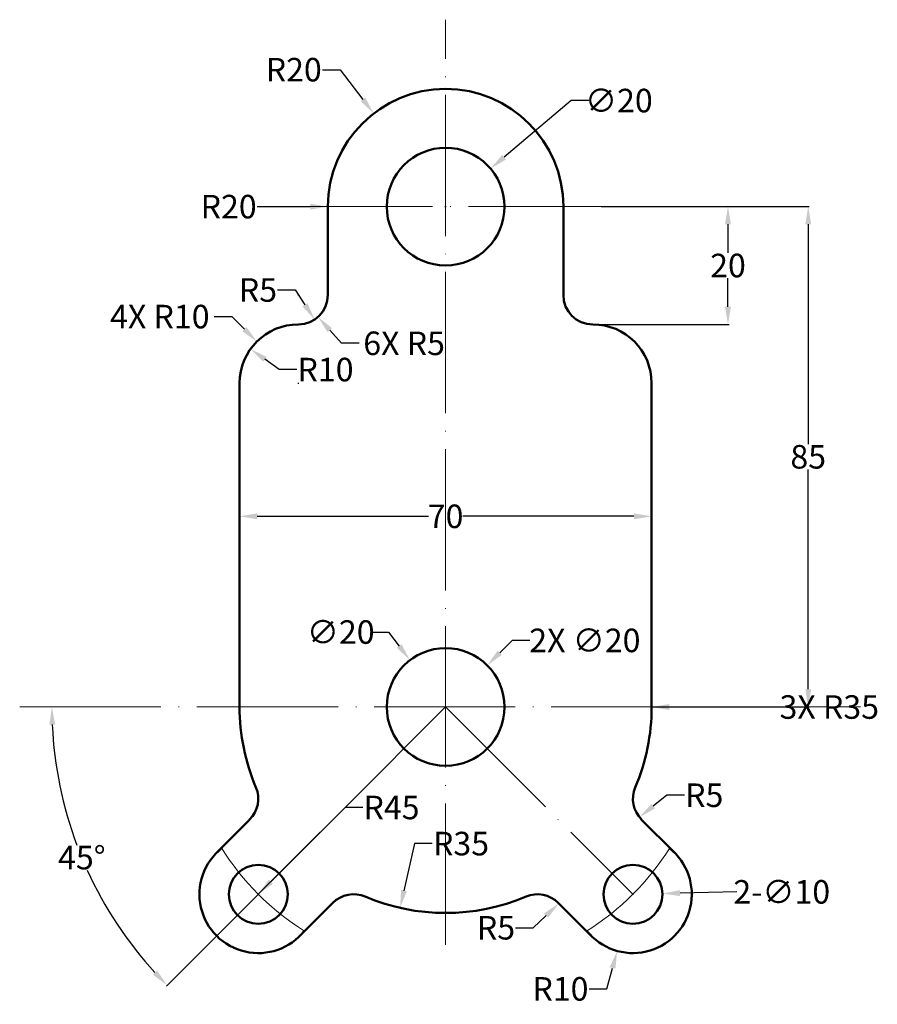
# Model space of a CAD drawing. Units: inches. Extents: x 93 to 239, y 45 to 212.
import ezdxf

# ---------------------------------------------------------------- set-up
doc = ezdxf.new("R2010")
doc.units = ezdxf.units.IN
doc.header["$MEASUREMENT"] = 0
doc.linetypes.add('ACAD_ISO04W100', pattern=[30, 24, -3, 0, -3])
for name, color, linetype, lineweight in [('M-CNTR', 4, 'ACAD_ISO04W100', 18), ('M-DIMS', 2, 'Continuous', 25), ('M-OUTL', 7, 'Continuous', 50)]:
    doc.layers.add(name, color=color, linetype=linetype, lineweight=lineweight)
doc.styles.get("Standard").update_dxf_attribs({"font": 'arial.ttf'})
doc.dimstyles.get("Standard").update_dxf_attribs({"dimtxt": 4, "dimasz": 3, "dimexe": 0.18, "dimexo": 0.0625, "dimgap": 0.09, "dimtad": 0, "dimtih": 1, "dimtoh": 1, "dimdec": 0, "dimzin": 0, "dimdsep": 46, "dimtxsty": 'Standard', "dimcen": 0.09, "dimadec": 0, "dimazin": 0, "dimtfac": 1, "dimtdec": 0, "dimtofl": 0, "dimtmove": 0, "dimatfit": 3, "dimfxl": 1, "dimtolj": 1, "dimtzin": 0, "dimarcsym": 0})

# ---------------------------------------------------------------- blocks, each defined once
blk = doc.blocks.new('*D1')
at = {"layer": 'Defpoints', "color": 0, "transparency": 16777216}
for p in [(192.05, 180.39), (190.67, 160.39), (213.64, 160.39)]:
    blk.add_point(p, dxfattribs=at)
at = {"layer": 'M-DIMS', "color": 0, "lineweight": -2, "transparency": 16777216}
for p, q in [((192.11, 180.39), (213.82, 180.39)), ((213.64, 177.39), (213.64, 172.53)), ((213.64, 163.39), (213.64, 168.26)), ((190.73, 160.39), (213.82, 160.39))]:
    blk.add_line(p, q, dxfattribs=at)
at = {"layer": 'M-DIMS', "color": 0, "transparency": 16777216}
for points in [[(213.14, 177.39), (214.14, 177.39), (213.64, 180.39)], [(213.14, 163.39), (214.14, 163.39), (213.64, 160.39)]]:
    blk.add_solid(points, dxfattribs=at)
at = {"layer": 'M-DIMS', "color": 0, "transparency": 16777216, "insert": (213.64, 170.39), "char_height": 4, "attachment_point": 5}
blk.add_mtext('\\A1;20', dxfattribs=at)
blk = doc.blocks.new('*D2')
at = {"layer": 'Defpoints', "color": 0, "transparency": 16777216}
for p in [(192.05, 180.39), (200.67, 95.39), (227.27, 95.39)]:
    blk.add_point(p, dxfattribs=at)
at = {"layer": 'M-DIMS', "color": 0, "lineweight": -2, "transparency": 16777216}
for p, q in [((192.11, 180.39), (227.45, 180.39)), ((227.27, 177.39), (227.27, 140.03)), ((227.27, 98.39), (227.27, 135.76)), ((200.73, 95.39), (227.45, 95.39))]:
    blk.add_line(p, q, dxfattribs=at)
at = {"layer": 'M-DIMS', "color": 0, "transparency": 16777216}
for points in [[(226.77, 177.39), (227.77, 177.39), (227.27, 180.39)], [(226.77, 98.39), (227.77, 98.39), (227.27, 95.39)]]:
    blk.add_solid(points, dxfattribs=at)
at = {"layer": 'M-DIMS', "color": 0, "transparency": 16777216, "insert": (227.27, 137.89), "char_height": 4, "attachment_point": 5}
blk.add_mtext('\\A1;85', dxfattribs=at)
blk = doc.blocks.new('*D3')
at = {"layer": 'Defpoints', "color": 0, "transparency": 16777216}
for p in [(197.49, 63.57), (194.82, 53.93)]:
    blk.add_point(p, dxfattribs=at)
at = {"layer": 'M-DIMS', "color": 0, "lineweight": -2, "transparency": 16777216}
for p, q in [((197.4, 63.57), (197.58, 63.57)), ((197.49, 63.48), (197.49, 63.66)), ((193.05, 47.5), (194.02, 51.04)), ((190.05, 47.5), (193.05, 47.5))]:
    blk.add_line(p, q, dxfattribs=at)
at = {"layer": 'M-DIMS', "color": 0, "transparency": 16777216}
blk.add_solid([(193.54, 51.18), (194.51, 50.91), (194.82, 53.93)], dxfattribs=at)
at = {"layer": 'M-DIMS', "color": 0, "transparency": 16777216, "insert": (185.18, 47.5), "char_height": 4, "attachment_point": 5}
blk.add_mtext('\\A1;R10', dxfattribs=at)
blk = doc.blocks.new('*D4')
at = {"layer": 'Defpoints', "color": 0, "transparency": 16777216}
for p in [(184.9, 62.02), (181.28, 58.57)]:
    blk.add_point(p, dxfattribs=at)
at = {"layer": 'M-DIMS', "color": 0, "lineweight": -2, "transparency": 16777216}
for p, q in [((180.56, 57.88), (182.73, 59.95)), ((177.56, 57.88), (180.56, 57.88))]:
    blk.add_line(p, q, dxfattribs=at)
blk.add_arc((181.28, 58.57), 5, 41.564, 44.2838, dxfattribs=at)
at = {"layer": 'M-DIMS', "color": 0, "transparency": 16777216}
blk.add_solid([(182.39, 60.31), (183.08, 59.58), (184.9, 62.02)], dxfattribs=at)
at = {"layer": 'M-DIMS', "color": 0, "transparency": 16777216, "insert": (174.23, 57.88), "char_height": 4, "attachment_point": 5}
blk.add_mtext('\\A1;R5', dxfattribs=at)
blk = doc.blocks.new('*D5')
at = {"layer": 'Defpoints', "color": 0, "transparency": 16777216}
for p in [(165.67, 95.39), (157.93, 61.26)]:
    blk.add_point(p, dxfattribs=at)
at = {"layer": 'M-DIMS', "color": 0, "lineweight": -2, "transparency": 16777216}
for p, q in [((160.41, 72.18), (158.59, 64.18)), ((163.41, 72.18), (160.41, 72.18))]:
    blk.add_line(p, q, dxfattribs=at)
at = {"layer": 'M-DIMS', "color": 0, "transparency": 16777216}
blk.add_solid([(158.11, 64.3), (159.08, 64.07), (157.93, 61.26)], dxfattribs=at)
at = {"layer": 'M-DIMS', "color": 0, "transparency": 16777216, "insert": (168.29, 72.18), "char_height": 4, "attachment_point": 5}
blk.add_mtext('\\A1;R35', dxfattribs=at)
blk = doc.blocks.new('*D6')
at = {"layer": 'Defpoints', "color": 0, "transparency": 16777216}
for p in [(202.49, 63.69), (192.49, 63.46)]:
    blk.add_point(p, dxfattribs=at)
at = {"layer": 'M-DIMS', "color": 0, "lineweight": -2, "transparency": 16777216}
for p, q in [((197.4, 63.57), (197.58, 63.57)), ((197.49, 63.48), (197.49, 63.66)), ((215.14, 63.98), (205.49, 63.76))]:
    blk.add_line(p, q, dxfattribs=at)
at = {"layer": 'M-DIMS', "color": 0, "transparency": 16777216}
blk.add_solid([(205.47, 64.26), (205.5, 63.26), (202.49, 63.69)], dxfattribs=at)
at = {"layer": 'M-DIMS', "color": 0, "transparency": 16777216, "insert": (222.78, 63.98), "char_height": 4, "attachment_point": 5}
blk.add_mtext('\\A1;2-∅10', dxfattribs=at)
blk = doc.blocks.new('*D7')
at = {"layer": 'Defpoints', "color": 0, "transparency": 16777216}
for p in [(202.5, 79.78), (198.58, 76.66)]:
    blk.add_point(p, dxfattribs=at)
at = {"layer": 'M-DIMS', "color": 0, "lineweight": -2, "transparency": 16777216}
for p, q in [((203.28, 80.4), (200.93, 78.53)), ((206.28, 80.4), (203.28, 80.4))]:
    blk.add_line(p, q, dxfattribs=at)
at = {"layer": 'M-DIMS', "color": 0, "transparency": 16777216}
blk.add_solid([(200.62, 78.92), (201.24, 78.14), (198.58, 76.66)], dxfattribs=at)
at = {"layer": 'M-DIMS', "color": 0, "transparency": 16777216, "insert": (209.61, 80.4), "char_height": 4, "attachment_point": 5}
blk.add_mtext('\\A1;R5', dxfattribs=at)
blk = doc.blocks.new('*D8')
at = {"layer": 'Defpoints', "color": 0, "transparency": 16777216}
for p in [(93.31, 95.39), (165.67, 95.39), (236.13, 95.39), (101.06, 78.08), (133.85, 63.57)]:
    blk.add_point(p, dxfattribs=at)
at = {"layer": 'M-DIMS', "color": 0, "lineweight": -2, "transparency": 16777216}
blk.add_line((133.8, 63.53), (118.24, 47.97), dxfattribs=at)
for start, end in [(182.5699, 200.5441), (204.484, 222.4301)]:
    blk.add_arc((165.67, 95.39), 66.89, start, end, dxfattribs=at)
at = {"layer": 'M-DIMS', "color": 0, "transparency": 16777216}
for points in [[(98.35, 92.38), (99.35, 92.4), (98.78, 95.39)], [(116.66, 50.61), (115.94, 49.92), (118.37, 48.09)]]:
    blk.add_solid(points, dxfattribs=at)
at = {"layer": 'M-DIMS', "color": 0, "transparency": 16777216, "insert": (103.87, 69.8), "char_height": 4, "attachment_point": 5}
blk.add_mtext('\\A1;45°', dxfattribs=at)
blk = doc.blocks.new('*D9')
at = {"layer": 'Defpoints', "color": 0, "transparency": 16777216}
for p in [(165.67, 95.39), (133.85, 63.57)]:
    blk.add_point(p, dxfattribs=at)
at = {"layer": 'M-DIMS', "color": 0, "lineweight": -2, "transparency": 16777216}
for p, q in [((148.59, 78.32), (135.97, 65.69)), ((151.59, 78.32), (148.59, 78.32))]:
    blk.add_line(p, q, dxfattribs=at)
at = {"layer": 'M-DIMS', "color": 0, "transparency": 16777216}
blk.add_solid([(135.62, 66.05), (136.32, 65.34), (133.85, 63.57)], dxfattribs=at)
at = {"layer": 'M-DIMS', "color": 0, "transparency": 16777216, "insert": (156.48, 78.32), "char_height": 4, "attachment_point": 5}
blk.add_mtext('\\A1;R45', dxfattribs=at)
blk = doc.blocks.new('*D10')
at = {"layer": 'Defpoints', "color": 0, "transparency": 16777216}
for p in [(159.61, 103.35), (171.73, 87.44)]:
    blk.add_point(p, dxfattribs=at)
at = {"layer": 'M-DIMS', "color": 0, "lineweight": -2, "transparency": 16777216}
for p, q in [((152.97, 108.12), (155.97, 108.12)), ((155.97, 108.12), (157.79, 105.73)), ((165.58, 95.39), (165.76, 95.39)), ((165.67, 95.3), (165.67, 95.48))]:
    blk.add_line(p, q, dxfattribs=at)
at = {"layer": 'M-DIMS', "color": 0, "transparency": 16777216}
blk.add_solid([(158.19, 106.04), (157.39, 105.43), (159.61, 103.35)], dxfattribs=at)
at = {"layer": 'M-DIMS', "color": 0, "transparency": 16777216, "insert": (147.85, 108.12), "char_height": 4, "attachment_point": 5}
blk.add_mtext('\\A1;∅20', dxfattribs=at)
blk = doc.blocks.new('*D11')
at = {"layer": 'Defpoints', "color": 0, "transparency": 16777216}
for p in [(200.67, 127.78), (130.67, 122.89), (200.67, 122.89)]:
    blk.add_point(p, dxfattribs=at)
at = {"layer": 'M-DIMS', "color": 0, "lineweight": -2, "transparency": 16777216}
for p, q in [((130.67, 122.96), (130.67, 127.96)), ((133.67, 127.78), (162.74, 127.78)), ((197.67, 127.78), (168.6, 127.78)), ((200.67, 122.96), (200.67, 127.96))]:
    blk.add_line(p, q, dxfattribs=at)
at = {"layer": 'M-DIMS', "color": 0, "transparency": 16777216}
for points in [[(133.67, 128.28), (133.67, 127.28), (130.67, 127.78)], [(197.67, 128.28), (197.67, 127.28), (200.67, 127.78)]]:
    blk.add_solid(points, dxfattribs=at)
at = {"layer": 'M-DIMS', "color": 0, "transparency": 16777216, "insert": (165.67, 127.78), "char_height": 4, "attachment_point": 5}
blk.add_mtext('\\A1;70', dxfattribs=at)
blk = doc.blocks.new('*D12')
at = {"layer": 'Defpoints', "color": 0, "transparency": 16777216}
for p in [(132.52, 156.19), (140.67, 150.39)]:
    blk.add_point(p, dxfattribs=at)
at = {"layer": 'M-DIMS', "color": 0, "lineweight": -2, "transparency": 16777216}
for p, q in [((137.41, 152.71), (134.97, 154.45)), ((140.41, 152.71), (137.41, 152.71))]:
    blk.add_line(p, q, dxfattribs=at)
at = {"layer": 'M-DIMS', "color": 0, "transparency": 16777216}
blk.add_solid([(135.26, 154.86), (134.68, 154.05), (132.52, 156.19)], dxfattribs=at)
at = {"layer": 'M-DIMS', "color": 0, "transparency": 16777216, "insert": (145.27, 152.71), "char_height": 4, "attachment_point": 5}
blk.add_mtext('\\A1;R10', dxfattribs=at)
blk = doc.blocks.new('*D13')
at = {"layer": 'Defpoints', "color": 0, "transparency": 16777216}
for p in [(140.67, 165.39), (143.42, 161.22)]:
    blk.add_point(p, dxfattribs=at)
at = {"layer": 'M-DIMS', "color": 0, "lineweight": -2, "transparency": 16777216}
for p, q in [((137.12, 166.23), (140.12, 166.23)), ((140.12, 166.23), (141.77, 163.72))]:
    blk.add_line(p, q, dxfattribs=at)
at = {"layer": 'M-DIMS', "color": 0, "transparency": 16777216}
blk.add_solid([(142.19, 164), (141.35, 163.45), (143.42, 161.22)], dxfattribs=at)
at = {"layer": 'M-DIMS', "color": 0, "transparency": 16777216, "insert": (133.79, 166.23), "char_height": 4, "attachment_point": 5}
blk.add_mtext('\\A1;R5', dxfattribs=at)
blk = doc.blocks.new('*D14')
at = {"layer": 'Defpoints', "color": 0, "transparency": 16777216}
for p in [(153.46, 196.23), (165.67, 180.39)]:
    blk.add_point(p, dxfattribs=at)
at = {"layer": 'M-DIMS', "color": 0, "lineweight": -2, "transparency": 16777216}
for p, q in [((144.73, 203.66), (147.73, 203.66)), ((147.73, 203.66), (151.63, 198.61)), ((165.58, 180.39), (165.76, 180.39)), ((165.67, 180.3), (165.67, 180.48))]:
    blk.add_line(p, q, dxfattribs=at)
at = {"layer": 'M-DIMS', "color": 0, "transparency": 16777216}
blk.add_solid([(152.02, 198.91), (151.23, 198.3), (153.46, 196.23)], dxfattribs=at)
at = {"layer": 'M-DIMS', "color": 0, "transparency": 16777216, "insert": (139.87, 203.66), "char_height": 4, "attachment_point": 5}
blk.add_mtext('\\A1;R20', dxfattribs=at)
blk = doc.blocks.new('*D15')
at = {"layer": 'Defpoints', "color": 0, "transparency": 16777216}
for p in [(173.31, 186.85), (158.03, 173.94)]:
    blk.add_point(p, dxfattribs=at)
at = {"layer": 'M-DIMS', "color": 0, "lineweight": -2, "transparency": 16777216}
for p, q in [((186.98, 198.41), (175.6, 188.78)), ((189.98, 198.41), (186.98, 198.41)), ((165.58, 180.39), (165.76, 180.39)), ((165.67, 180.3), (165.67, 180.48))]:
    blk.add_line(p, q, dxfattribs=at)
at = {"layer": 'M-DIMS', "color": 0, "transparency": 16777216}
blk.add_solid([(175.27, 189.17), (175.92, 188.4), (173.31, 186.85)], dxfattribs=at)
at = {"layer": 'M-DIMS', "color": 0, "transparency": 16777216, "insert": (195.1, 198.41), "char_height": 4, "attachment_point": 5}
blk.add_mtext('\\A1;∅20', dxfattribs=at)
blk = doc.blocks.new('*D16')
at = {"layer": 'Defpoints', "color": 0, "transparency": 16777216}
for p in [(145.67, 180.39), (165.67, 180.39)]:
    blk.add_point(p, dxfattribs=at)
at = {"layer": 'M-DIMS', "color": 0, "lineweight": -2, "transparency": 16777216}
for p, q in [((133.67, 180.39), (142.67, 180.39)), ((165.58, 180.39), (165.76, 180.39)), ((165.67, 180.3), (165.67, 180.48))]:
    blk.add_line(p, q, dxfattribs=at)
at = {"layer": 'M-DIMS', "color": 0, "transparency": 16777216}
blk.add_solid([(142.67, 180.89), (142.67, 179.89), (145.67, 180.39)], dxfattribs=at)
at = {"layer": 'M-DIMS', "color": 0, "transparency": 16777216, "insert": (128.81, 180.39), "char_height": 4, "attachment_point": 5}
blk.add_mtext('\\A1;R20', dxfattribs=at)
blk = doc.blocks.new('*D17')
at = {"layer": 'Defpoints', "color": 0, "transparency": 16777216}
for p in [(172.74, 102.46), (158.6, 88.32)]:
    blk.add_point(p, dxfattribs=at)
at = {"layer": 'M-DIMS', "color": 0, "lineweight": -2, "transparency": 16777216}
for p, q in [((176.99, 106.7), (174.86, 104.58)), ((179.99, 106.7), (176.99, 106.7)), ((165.58, 95.39), (165.76, 95.39)), ((165.67, 95.3), (165.67, 95.48))]:
    blk.add_line(p, q, dxfattribs=at)
at = {"layer": 'M-DIMS', "color": 0, "transparency": 16777216}
blk.add_solid([(174.51, 104.94), (175.22, 104.23), (172.74, 102.46)], dxfattribs=at)
at = {"layer": 'M-DIMS', "color": 0, "transparency": 16777216, "insert": (189.33, 106.7), "char_height": 4, "attachment_point": 5}
blk.add_mtext('\\A1;2X ∅20', dxfattribs=at)
blk = doc.blocks.new('*D18')
at = {"layer": 'Defpoints', "color": 0, "transparency": 16777216}
for p in [(133.6, 157.46), (140.67, 150.39)]:
    blk.add_point(p, dxfattribs=at)
at = {"layer": 'M-DIMS', "color": 0, "lineweight": -2, "transparency": 16777216}
for p, q in [((126.36, 161.71), (129.36, 161.71)), ((129.36, 161.71), (131.48, 159.59)), ((140.58, 150.39), (140.76, 150.39)), ((140.67, 150.3), (140.67, 150.48))]:
    blk.add_line(p, q, dxfattribs=at)
at = {"layer": 'M-DIMS', "color": 0, "transparency": 16777216}
blk.add_solid([(131.83, 159.94), (131.12, 159.23), (133.6, 157.46)], dxfattribs=at)
at = {"layer": 'M-DIMS', "color": 0, "transparency": 16777216, "insert": (117.12, 161.71), "char_height": 4, "attachment_point": 5}
blk.add_mtext('\\A1;4X R10', dxfattribs=at)
blk = doc.blocks.new('*D19')
at = {"layer": 'Defpoints', "color": 0, "transparency": 16777216}
for p in [(140.67, 165.39), (143.99, 161.66)]:
    blk.add_point(p, dxfattribs=at)
at = {"layer": 'M-DIMS', "color": 0, "lineweight": -2, "transparency": 16777216}
for p, q in [((140.58, 165.39), (140.76, 165.39)), ((140.67, 165.3), (140.67, 165.48)), ((147.98, 157.17), (145.98, 159.41)), ((150.98, 157.17), (147.98, 157.17))]:
    blk.add_line(p, q, dxfattribs=at)
at = {"layer": 'M-DIMS', "color": 0, "transparency": 16777216}
blk.add_solid([(146.36, 159.75), (145.61, 159.08), (143.99, 161.66)], dxfattribs=at)
at = {"layer": 'M-DIMS', "color": 0, "transparency": 16777216, "insert": (158.62, 157.17), "char_height": 4, "attachment_point": 5}
blk.add_mtext('\\A1;6X R5', dxfattribs=at)
blk = doc.blocks.new('*D20')
at = {"layer": 'Defpoints', "color": 0, "transparency": 16777216}
for p in [(165.67, 95.39), (200.67, 95.38)]:
    blk.add_point(p, dxfattribs=at)
at = {"layer": 'M-DIMS', "color": 0, "lineweight": -2, "transparency": 16777216}
for p, q in [((165.58, 95.39), (165.76, 95.39)), ((165.67, 95.3), (165.67, 95.48)), ((221.67, 95.38), (203.67, 95.38))]:
    blk.add_line(p, q, dxfattribs=at)
at = {"layer": 'M-DIMS', "color": 0, "transparency": 16777216}
blk.add_solid([(203.67, 95.88), (203.67, 94.88), (200.67, 95.38)], dxfattribs=at)
at = {"layer": 'M-DIMS', "color": 0, "transparency": 16777216, "insert": (230.85, 95.38), "char_height": 4, "attachment_point": 5}
blk.add_mtext('\\A1;3X R35', dxfattribs=at)

msp = doc.modelspace()

# ---------------------------------------------------------------- linework, layer by layer
at = {"layer": 'M-CNTR'}
for p, q in [((165.67, 54.99), (165.67, 212.15)), ((139.45, 180.39), (192.05, 180.39)), ((93.31, 95.39), (236.13, 95.39)), ((165.67, 95.39), (133.85, 63.57)), ((165.67, 95.39), (197.49, 63.57))]:
    msp.add_line(p, q, dxfattribs=at)
for start, end in [(212.1604, 237.8396), (302.1604, 327.8396)]:
    msp.add_arc((165.67, 95.39), 45, start, end, dxfattribs=at)
at = {"layer": 'M-OUTL'}
for p, q in [((145.67, 180.39), (145.67, 165.39)), ((185.67, 180.39), (185.67, 165.39)), ((140.67, 160.39), (140.67, 160.39)), ((190.67, 160.39), (190.67, 160.39)), ((130.67, 95.39), (130.67, 150.39)), ((200.67, 95.39), (200.67, 150.39)), ((126.78, 70.64), (132.38, 76.24)), ((204.56, 70.64), (198.96, 76.24)), ((140.92, 56.5), (146.52, 62.1)), ((190.42, 56.5), (184.82, 62.1))]:
    msp.add_line(p, q, dxfattribs=at)
for centre, radius in [((165.67, 180.39), 10), ((165.67, 95.39), 10), ((133.85, 63.57), 5), ((197.49, 63.57), 5)]:
    msp.add_circle(centre, radius, dxfattribs=at)
for centre, radius, start, end in [((165.67, 180.39), 20, 0, 180), ((140.67, 165.39), 5, 270, 0), ((190.67, 165.39), 5, 180, 270), ((140.67, 150.39), 10, 90, 180), ((190.67, 150.39), 10, 0, 90), ((165.67, 95.39), 35, 180, 202.9757), ((165.67, 95.39), 35, 337.0243, 0), ((128.84, 79.78), 5, 315, 22.9757), ((202.5, 79.78), 5, 157.0243, 225), ((133.85, 63.57), 10, 128.6206, 321.3794), ((197.49, 63.57), 10, 218.6206, 51.3794), ((150.06, 58.57), 5, 67.0243, 135), ((181.28, 58.57), 5, 45, 112.9757), ((165.67, 95.39), 35, 247.0243, 292.9757)]:
    msp.add_arc(centre, radius, start, end, dxfattribs=at)

# ---------------------------------------------------------------- dimensions: what is measured, and where the dimension line sits
at = {"layer": 'M-DIMS'}
for center, mpoint, override, picture, middle in [((165.67, 180.39), (153.46, 196.23), {"dimclrd": 0, "dimclre": 0, "dimclrt": 0}, '*D14', (139.87, 203.66)), ((165.67, 180.39), (145.67, 180.39), {"dimdec": 0, "dimlfac": 1, "dimrnd": 0, "dimzin": 0, "dimdsep": 46, "dimlunit": 2}, '*D16', (133.67, 180.39)), ((140.67, 165.39), (143.42, 161.22), {"dimclrd": 0, "dimclre": 0, "dimclrt": 0}, '*D13', (133.79, 166.23)), ((140.67, 150.39), (132.52, 156.19), {"dimclrd": 0, "dimclre": 0, "dimclrt": 0}, '*D12', (145.27, 152.71)), ((165.67, 95.39), (133.85, 63.57), {"dimclrd": 0, "dimclre": 0, "dimclrt": 0}, '*D9', (156.48, 78.32)), ((165.67, 95.39), (157.93, 61.26), {"dimclrd": 0, "dimclre": 0, "dimclrt": 0}, '*D5', (168.29, 72.18)), ((202.5, 79.78), (198.58, 76.66), {"dimclrd": 0, "dimclre": 0, "dimclrt": 0}, '*D7', (209.61, 80.4)), ((197.49, 63.57), (194.82, 53.93), {"dimclrd": 0, "dimclre": 0, "dimclrt": 0}, '*D3', (185.18, 47.5)), ((181.28, 58.57), (184.9, 62.02), {"dimclrd": 0, "dimclre": 0, "dimclrt": 0}, '*D4', (174.23, 57.88))]:
    dim = msp.add_radius_dim(center=center, mpoint=mpoint, dimstyle='Standard', override=override, dxfattribs=at)
    dim.commit()
    dim.dimension.update_dxf_attribs({"geometry": picture, "text_midpoint": middle, "dimtype": 164})
for p1, p2, picture, middle in [((158.03, 173.94), (173.31, 186.85), '*D15', (195.1, 198.41)), ((171.73, 87.44), (159.61, 103.35), '*D10', (147.85, 108.12))]:
    dim = msp.add_diameter_dim_2p(p1=p1, p2=p2, dimstyle='Standard', override={"dimclrd": 0, "dimclre": 0, "dimclrt": 0}, dxfattribs=at)
    dim.commit()
    dim.dimension.update_dxf_attribs({"geometry": picture, "text_midpoint": middle, "dimtype": 163})
for base, p2, picture, middle in [((213.64, 160.39), (190.67, 160.39), '*D1', (213.64, 170.39)), ((227.27, 95.39), (200.67, 95.39), '*D2', (227.27, 137.89))]:
    dim = msp.add_linear_dim(base=base, p1=(192.05, 180.39), p2=p2, angle=90, dimstyle='Standard', override={"dimclrd": 0, "dimclre": 0, "dimclrt": 0}, dxfattribs=at)
    dim.commit()
    dim.dimension.update_dxf_attribs({"geometry": picture, "text_midpoint": middle})
for center, mpoint, text, picture, middle in [((140.67, 150.39), (133.6, 157.46), '4X <>', '*D18', (117.12, 161.71)), ((165.67, 95.39), (200.67, 95.38), '3X <>', '*D20', (221.67, 95.38))]:
    dim = msp.add_radius_dim(center=center, mpoint=mpoint, text=text, dimstyle='Standard', override={"dimdec": 0, "dimlfac": 1, "dimrnd": 0, "dimzin": 0, "dimdsep": 46, "dimlunit": 2}, dxfattribs=at)
    dim.commit()
    dim.dimension.update_dxf_attribs({"geometry": picture, "text_midpoint": middle, "dimtype": 164})
dim = msp.add_radius_dim(center=(140.67, 165.39), mpoint=(143.99, 161.66), text='6X <>', dimstyle='Standard', override={"dimdec": 0, "dimlfac": 1, "dimrnd": 0, "dimzin": 0, "dimdsep": 46, "dimlunit": 2}, dxfattribs=at)
dim.commit()
dim.dimension.update_dxf_attribs({"geometry": '*D19', "text_midpoint": (158.62, 157.17)})
dim = msp.add_linear_dim(base=(200.67, 127.78), p1=(130.67, 122.89), p2=(200.67, 122.89), dimstyle='Standard', override={"dimclrd": 0, "dimclre": 0, "dimclrt": 0}, dxfattribs=at)
dim.commit()
dim.dimension.update_dxf_attribs({"geometry": '*D11', "text_midpoint": (165.67, 127.78)})
for p1, p2, text, override, picture, middle in [((158.6, 88.32), (172.74, 102.46), '2X <>', {"dimdec": 0, "dimlfac": 1, "dimrnd": 0, "dimzin": 0, "dimdsep": 46, "dimlunit": 2}, '*D17', (189.33, 106.7)), ((192.49, 63.46), (202.49, 63.69), '2-<>', {"dimclrd": 0, "dimclre": 0, "dimclrt": 0}, '*D6', (215.14, 63.98))]:
    dim = msp.add_diameter_dim_2p(p1=p1, p2=p2, text=text, dimstyle='Standard', override=override, dxfattribs=at)
    dim.commit()
    dim.dimension.update_dxf_attribs({"geometry": picture, "text_midpoint": middle, "dimtype": 163})
dim = msp.add_angular_dim_2l(base=(101.06, 78.08), line1=((93.31, 95.39), (236.13, 95.39)), line2=((165.67, 95.39), (133.85, 63.57)), dimstyle='Standard', override={"dimclrd": 0, "dimclre": 0, "dimclrt": 0}, dxfattribs=at)
dim.commit()
dim.dimension.update_dxf_attribs({"geometry": '*D8', "text_midpoint": (103.87, 69.8)})

doc.saveas('drawing.dxf')
